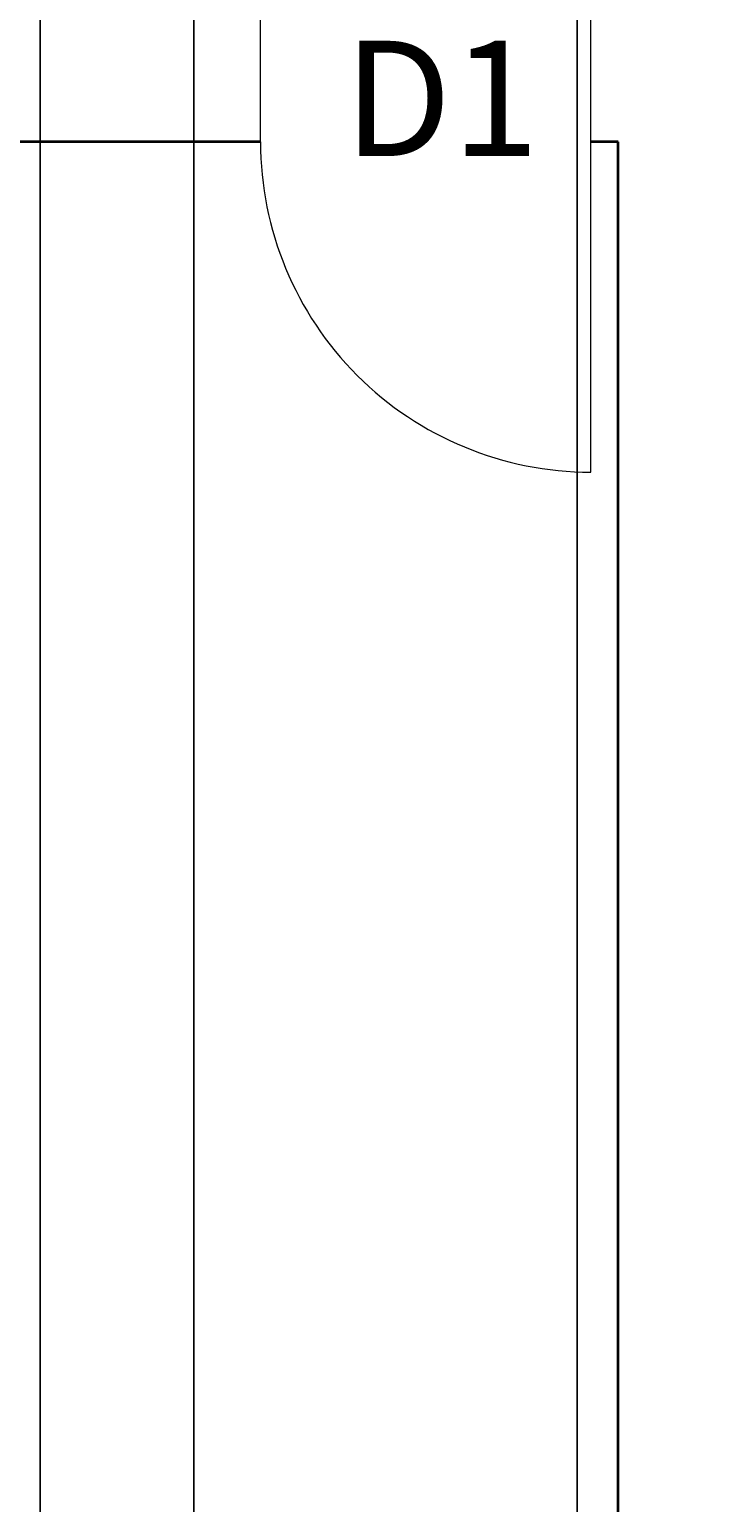
# Model space of a CAD drawing. Units: feet. Extents: x 1654 to 2985, y 1348 to 2230.
# Tile 14 of 53: x 1956 to 2007, y 1643 to 1750. Entities that reach past the tile are written whole.
import ezdxf

# ---------------------------------------------------------------- set-up
doc = ezdxf.new("R2010")
doc.units = ezdxf.units.FT
for name, color, linetype, lineweight in [('A-ANNO-DIMS', 2, 'Continuous', 18), ('A-ANNO-TEXT', 7, 'Continuous', 18), ('A-DOOR', 3, 'Continuous', 18), ('A-WALL', 7, 'Continuous', 35)]:
    doc.layers.add(name, color=color, linetype=linetype, lineweight=lineweight)
doc.styles.get("Standard").update_dxf_attribs({"font": 'arial.ttf'})
doc.dimstyles.get("Standard").update_dxf_attribs({"dimtxt": 0.18, "dimasz": 0.18, "dimexe": 0.18, "dimexo": 0.0625, "dimgap": 0.09, "dimtad": 0, "dimtih": 1, "dimtoh": 1, "dimdec": 4, "dimzin": 0, "dimdsep": 46, "dimtxsty": 'Standard', "dimcen": 0.09, "dimadec": 0, "dimazin": 0, "dimtfac": 1, "dimtdec": 4, "dimtofl": 0, "dimtmove": 0, "dimatfit": 3, "dimfxl": 1, "dimtolj": 1, "dimtzin": 0, "dimarcsym": 0})

# ---------------------------------------------------------------- blocks, each defined once
blk = doc.blocks.new('DOOR-INT-SINGLE')
for p, q in [((0, 24), (9, 24)), ((-24, 0), (9, 0))]:
    blk.add_line(p, q)
blk.add_arc((0, 0), 24, 90, 180)
blk = doc.blocks.new('*D97')
at = {"layer": 'A-ANNO-DIMS', "color": 0, "lineweight": -2, "transparency": 16777216}
for p, q in [((1957.09, 2108.19), (1957.09, 1534.07)), ((1968.25, 2108.19), (1968.25, 1534.07)), ((1957.27, 1534.25), (1962.22, 1534.25)), ((1968.07, 1534.25), (1963.13, 1534.25))]:
    blk.add_line(p, q, dxfattribs=at)
at = {"layer": 'A-ANNO-DIMS', "color": 0, "transparency": 16777216}
for points in [[(1957.27, 1534.28), (1957.27, 1534.22), (1957.09, 1534.25)], [(1968.07, 1534.28), (1968.07, 1534.22), (1968.25, 1534.25)]]:
    blk.add_solid(points, dxfattribs=at)
at = {"layer": 'Defpoints', "color": 0, "transparency": 16777216}
for p in [(1957.09, 2108.25), (1968.25, 2108.25), (1968.25, 1534.25)]:
    blk.add_point(p, dxfattribs=at)
at = {"layer": 'A-ANNO-DIMS', "color": 0, "transparency": 16777216, "insert": (1962.67, 1534.25), "char_height": 0.18, "attachment_point": 5}
blk.add_mtext('\\A1;11.162', dxfattribs=at)
blk = doc.blocks.new('*D101')
at = {"layer": 'A-ANNO-DIMS', "color": 0, "lineweight": -2, "transparency": 16777216}
for p, q in [((1996.09, 2039.19), (1996.09, 1534.07)), ((2014.02, 2039.19), (2014.02, 1534.07)), ((1996.27, 1534.25), (2004.6, 1534.25)), ((2013.84, 1534.25), (2005.51, 1534.25))]:
    blk.add_line(p, q, dxfattribs=at)
at = {"layer": 'A-ANNO-DIMS', "color": 0, "transparency": 16777216}
for points in [[(1996.27, 1534.28), (1996.27, 1534.22), (1996.09, 1534.25)], [(2013.84, 1534.28), (2013.84, 1534.22), (2014.02, 1534.25)]]:
    blk.add_solid(points, dxfattribs=at)
at = {"layer": 'Defpoints', "color": 0, "transparency": 16777216}
for p in [(1996.09, 2039.25), (2014.02, 2039.25), (2014.02, 1534.25)]:
    blk.add_point(p, dxfattribs=at)
at = {"layer": 'A-ANNO-DIMS', "color": 0, "transparency": 16777216, "insert": (2005.05, 1534.25), "char_height": 0.18, "attachment_point": 5}
blk.add_mtext('\\A1;17.924', dxfattribs=at)

msp = doc.modelspace()

# ---------------------------------------------------------------- linework, layer by layer
at = {"layer": 'A-WALL'}
for p, q in [((1973.0924, 1742.2549), (1948.0924, 1742.2549)), ((1999.0924, 1742.2549), (1997.0924, 1742.2549)), ((1999.0924, 1600.2549), (1999.0924, 1742.2549))]:
    msp.add_line(p, q, dxfattribs=at)

# ---------------------------------------------------------------- block references
at = {"layer": 'A-DOOR', "rotation": 90.00000000000055}
msp.add_blockref('DOOR-INT-SINGLE', (1997.0924, 1742.2549), dxfattribs=at)

# ---------------------------------------------------------------- texts
at = {"layer": 'A-ANNO-TEXT'}
msp.add_text('D1', height=8.38114, dxfattribs=at).set_placement((1979.1211, 1741.2317))

# ---------------------------------------------------------------- dimensions: what is measured, and where the dimension line sits
at = {"layer": 'A-ANNO-DIMS'}
for base, p1, p2, picture, middle in [((1968.2542, 1534.2549), (1957.0924, 2108.2549), (1968.2542, 2108.2549), '*D97', (1962.6733, 1534.2549)), ((2014.016, 1534.2549), (1996.0924, 2039.2549), (2014.016, 2039.2549), '*D101', (2005.0542, 1534.2549))]:
    dim = msp.add_linear_dim(base=base, p1=p1, p2=p2, dimstyle='Standard', override={"dimdec": 3, "dimlfac": 1, "dimrnd": 0, "dimzin": 0, "dimdsep": 46, "dimlunit": 2}, dxfattribs=at)
    dim.commit()
    dim.dimension.update_dxf_attribs({"geometry": picture, "text_midpoint": middle})

doc.saveas('drawing.dxf')
